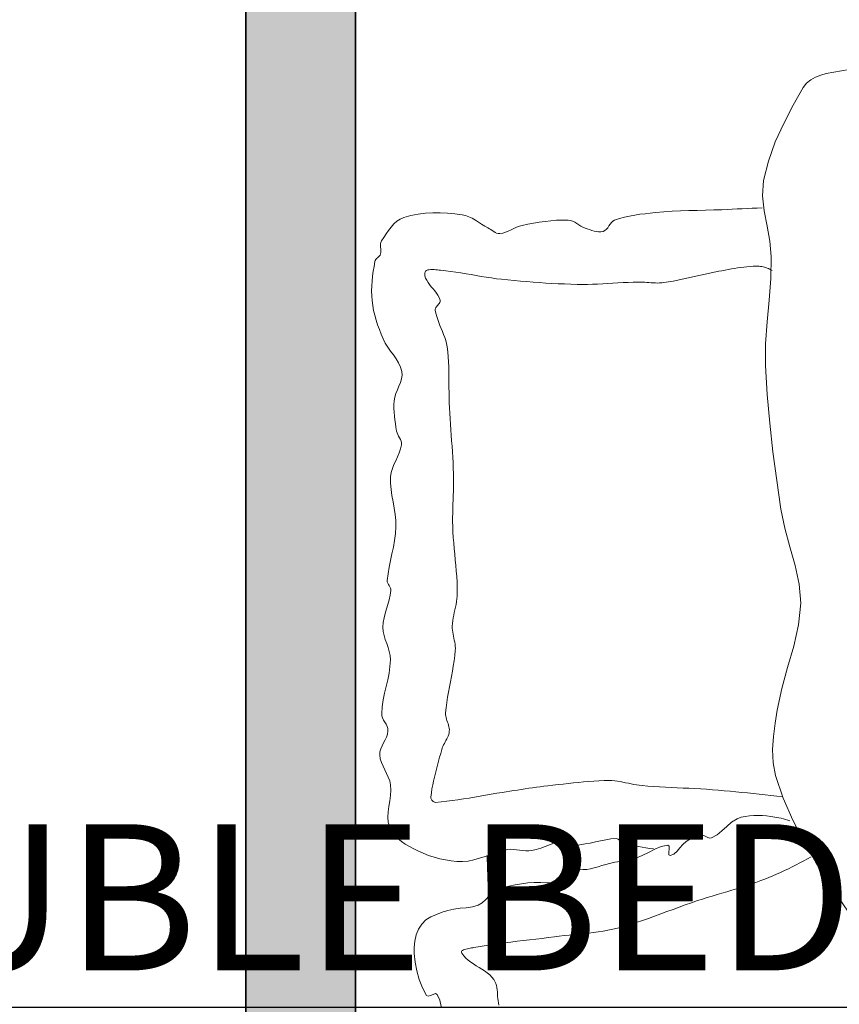
# Model space of a CAD drawing. Units: inches. Extents: x 2656 to 9931, y 1941 to 3068.
# Tile 16 of 46: x 2863 to 2896, y 2490 to 2530. Entities that reach past the tile are written whole.
import ezdxf

# ---------------------------------------------------------------- set-up
doc = ezdxf.new("R2010")
doc.units = ezdxf.units.IN
for name, color, linetype, lineweight in [('A-ANNO-DIMS', 2, 'Continuous', 18), ('A-FURN', 8, 'Continuous', 13), ('A-WALL', 7, 'Continuous', 35), ('A-WALL-PATT', 251, 'Continuous', 13)]:
    doc.layers.add(name, color=color, linetype=linetype, lineweight=lineweight)
doc.styles.get("Standard").update_dxf_attribs({"font": 'arial.ttf'})
doc.dimstyles.new('ISO-25', dxfattribs={"dimtxt": 6, "dimasz": 2.5, "dimexe": 1.25, "dimexo": 0.625, "dimtad": 1, "dimdec": 0, "dimlunit": 3, "dimtxsty": 'Standard', "dimcen": 2.5, "dimadec": 0, "dimazin": 0, "dimtfac": 1, "dimtdec": 0, "dimtmove": 0, "dimatfit": 3, "dimfxl": 1, "dimarcsym": 0})

# ---------------------------------------------------------------- blocks, each defined once
blk = doc.blocks.new('BED-DOUBLE')
for p, q in [((19.868, 60.758), (18.612, 60.54)), ((17.974, 60.285), (17.799, 60.142)), ((18.176, 60.399), (17.974, 60.285)), ((18.392, 60.483), (18.176, 60.399)), ((18.612, 60.54), (18.392, 60.483)), ((17.664, 59.967), (17.251, 59.242)), ((17.799, 60.142), (17.664, 59.967)), ((17.251, 59.242), (16.864, 58.499)), ((16.864, 58.499), (16.52, 57.736)), ((16.52, 57.736), (16.239, 56.953)), ((16.239, 56.953), (16.039, 56.149)), ((16.039, 56.149), (15.997, 55.53)), ((15.997, 55.53), (16.064, 54.908)), ((14.539, 54.965), (14.333, 54.956)), ((14.745, 54.974), (14.539, 54.965)), ((14.951, 54.984), (14.745, 54.974)), ((15.157, 54.993), (14.951, 54.984)), ((15.363, 55.002), (15.157, 54.993)), ((15.569, 55.012), (15.363, 55.002)), ((15.775, 55.021), (15.569, 55.012)), ((15.98, 55.031), (15.775, 55.021)), ((1.134, 54.573), (0.997, 54.482)), ((1.286, 54.638), (1.134, 54.573)), ((1.573, 54.718), (1.286, 54.638)), ((1.867, 54.773), (1.573, 54.718)), ((2.165, 54.807), (1.867, 54.773)), ((2.466, 54.823), (2.165, 54.807)), ((2.769, 54.822), (2.466, 54.823)), ((3.071, 54.807), (2.769, 54.822)), ((3.373, 54.782), (3.071, 54.807)), ((3.671, 54.748), (3.373, 54.782)), ((3.815, 54.718), (3.671, 54.748)), ((3.953, 54.668), (3.815, 54.718)), ((4.086, 54.602), (3.953, 54.668)), ((4.216, 54.525), (4.086, 54.602)), ((10.131, 54.589), (9.929, 54.522)), ((10.337, 54.645), (10.131, 54.589)), ((10.545, 54.692), (10.337, 54.645)), ((10.755, 54.732), (10.545, 54.692)), ((10.967, 54.765), (10.755, 54.732)), ((11.179, 54.792), (10.967, 54.765)), ((11.392, 54.817), (11.179, 54.792)), ((11.605, 54.838), (11.392, 54.817)), ((11.945, 54.867), (11.605, 54.838)), ((12.285, 54.889), (11.945, 54.867)), ((12.626, 54.904), (12.285, 54.889)), ((12.968, 54.916), (12.626, 54.904)), ((13.309, 54.925), (12.968, 54.916)), ((13.651, 54.933), (13.309, 54.925)), ((13.992, 54.943), (13.651, 54.933)), ((14.333, 54.956), (13.992, 54.943)), ((16.064, 54.908), (16.183, 54.283)), ((0.756, 54.244), (0.65, 54.106)), ((0.871, 54.371), (0.756, 54.244)), ((0.997, 54.482), (0.871, 54.371)), ((4.344, 54.443), (4.216, 54.525)), ((4.471, 54.359), (4.344, 54.443)), ((4.6, 54.279), (4.471, 54.359)), ((4.732, 54.207), (4.6, 54.279)), ((4.791, 54.174), (4.732, 54.207)), ((4.85, 54.136), (4.791, 54.174)), ((5.792, 54.184), (5.68, 54.13)), ((5.905, 54.235), (5.792, 54.184)), ((6.02, 54.279), (5.905, 54.235)), ((6.138, 54.31), (6.02, 54.279)), ((6.371, 54.355), (6.138, 54.31)), ((6.605, 54.399), (6.371, 54.355)), ((6.84, 54.439), (6.605, 54.399)), ((7.076, 54.474), (6.84, 54.439)), ((7.312, 54.503), (7.076, 54.474)), ((7.548, 54.522), (7.312, 54.503)), ((7.785, 54.531), (7.548, 54.522)), ((8.022, 54.528), (7.785, 54.531)), ((8.115, 54.514), (8.022, 54.528)), ((8.204, 54.483), (8.115, 54.514)), ((8.29, 54.44), (8.204, 54.483)), ((8.374, 54.39), (8.29, 54.44)), ((8.458, 54.336), (8.374, 54.39)), ((8.542, 54.284), (8.458, 54.336)), ((8.628, 54.237), (8.542, 54.284)), ((8.717, 54.201), (8.628, 54.237)), ((8.808, 54.17), (8.717, 54.201)), ((8.9, 54.138), (8.808, 54.17)), ((9.647, 54.214), (9.593, 54.149)), ((9.696, 54.287), (9.647, 54.214)), ((9.746, 54.36), (9.696, 54.287)), ((9.799, 54.428), (9.746, 54.36)), ((9.858, 54.484), (9.799, 54.428)), ((9.929, 54.522), (9.858, 54.484)), ((16.183, 54.283), (16.3, 53.657)), ((0.456, 53.815), (0.365, 53.671)), ((0.55, 53.961), (0.456, 53.815)), ((0.65, 54.106), (0.55, 53.961)), ((4.909, 54.096), (4.85, 54.136)), ((4.968, 54.058), (4.909, 54.096)), ((5.028, 54.024), (4.968, 54.058)), ((5.089, 53.997), (5.028, 54.024)), ((5.153, 53.981), (5.089, 53.997)), ((5.218, 53.978), (5.153, 53.981)), ((5.338, 53.997), (5.218, 53.978)), ((5.454, 54.031), (5.338, 53.997)), ((5.568, 54.077), (5.454, 54.031)), ((5.68, 54.13), (5.568, 54.077)), ((8.993, 54.107), (8.9, 54.138)), ((9.087, 54.08), (8.993, 54.107)), ((9.181, 54.059), (9.087, 54.08)), ((9.274, 54.048), (9.181, 54.059)), ((9.367, 54.049), (9.274, 54.048)), ((9.459, 54.064), (9.367, 54.049)), ((9.532, 54.097), (9.459, 54.064)), ((9.593, 54.149), (9.532, 54.097)), ((0.326, 53.548), (0.324, 53.481)), ((0.324, 53.481), (0.33, 53.412)), ((0.337, 53.612), (0.326, 53.548)), ((0.33, 53.412), (0.337, 53.342)), ((0.365, 53.671), (0.337, 53.612)), ((16.3, 53.657), (16.356, 53.03)), ((0.167, 52.946), (0.134, 52.909)), ((0.203, 52.982), (0.167, 52.946)), ((0.241, 53.017), (0.203, 52.982)), ((0.276, 53.054), (0.241, 53.017)), ((0.306, 53.094), (0.276, 53.054)), ((0.326, 53.138), (0.306, 53.094)), ((0.339, 53.203), (0.326, 53.138)), ((0.337, 53.342), (0.341, 53.272)), ((0.341, 53.272), (0.339, 53.203)), ((16.356, 53.03), (16.332, 52.135)), ((0.058, 52.625), (0.027, 52.426)), ((0.093, 52.823), (0.058, 52.625)), ((0.108, 52.868), (0.093, 52.823)), ((0.134, 52.909), (0.108, 52.868)), ((14.717, 52.521), (14.845, 52.543)), ((14.845, 52.543), (14.973, 52.563)), ((14.973, 52.563), (15.102, 52.582)), ((15.102, 52.582), (15.23, 52.599)), ((15.23, 52.599), (15.359, 52.614)), ((15.359, 52.614), (15.488, 52.625)), ((15.488, 52.625), (15.617, 52.633)), ((15.617, 52.633), (15.747, 52.637)), ((15.747, 52.637), (15.802, 52.637)), ((15.802, 52.637), (15.858, 52.634)), ((15.858, 52.634), (15.913, 52.628)), ((15.913, 52.628), (15.969, 52.619)), ((15.969, 52.619), (16.024, 52.608)), ((16.024, 52.608), (16.079, 52.595)), ((16.079, 52.595), (16.133, 52.579)), ((16.133, 52.579), (16.186, 52.561)), ((16.186, 52.561), (16.238, 52.54)), ((16.238, 52.54), (16.289, 52.517)), ((0, 52.226), (-0.022, 52.025)), ((0.027, 52.426), (0, 52.226)), ((2.14, 52.349), (2.15, 52.398)), ((2.149, 52.246), (2.14, 52.349)), ((2.176, 52.149), (2.149, 52.246)), ((2.15, 52.398), (2.175, 52.435)), ((2.175, 52.435), (2.213, 52.463)), ((2.219, 52.056), (2.176, 52.149)), ((2.213, 52.463), (2.262, 52.481)), ((2.262, 52.481), (2.32, 52.492)), ((2.32, 52.492), (2.384, 52.497)), ((2.384, 52.497), (2.453, 52.497)), ((2.453, 52.497), (2.525, 52.494)), ((2.525, 52.494), (2.597, 52.487)), ((2.597, 52.487), (2.666, 52.48)), ((2.666, 52.48), (2.731, 52.473)), ((2.731, 52.473), (2.79, 52.468)), ((2.79, 52.468), (3, 52.448)), ((3, 52.448), (3.209, 52.423)), ((3.209, 52.423), (3.417, 52.394)), ((3.417, 52.394), (3.625, 52.362)), ((3.625, 52.362), (3.833, 52.327)), ((3.833, 52.327), (4.041, 52.291)), ((4.041, 52.291), (4.248, 52.254)), ((4.248, 52.254), (4.456, 52.218)), ((4.456, 52.218), (4.664, 52.184)), ((4.664, 52.184), (4.872, 52.152)), ((4.872, 52.152), (5.081, 52.123)), ((12.705, 52.097), (12.892, 52.139)), ((12.892, 52.139), (13.08, 52.182)), ((13.08, 52.182), (13.267, 52.226)), ((13.267, 52.226), (13.454, 52.269)), ((13.454, 52.269), (13.641, 52.312)), ((13.641, 52.312), (13.829, 52.354)), ((13.829, 52.354), (14.017, 52.392)), ((14.017, 52.392), (14.206, 52.428)), ((14.206, 52.428), (14.333, 52.451)), ((14.333, 52.451), (14.461, 52.474)), ((14.461, 52.474), (14.589, 52.498)), ((14.589, 52.498), (14.717, 52.521)), ((16.332, 52.135), (16.264, 51.241)), ((16.289, 52.517), (16.338, 52.491)), ((16.338, 52.491), (16.386, 52.464)), ((-0.036, 51.824), (-0.042, 51.623)), ((-0.022, 52.025), (-0.036, 51.824)), ((2.274, 51.966), (2.219, 52.056)), ((2.338, 51.878), (2.274, 51.966)), ((2.408, 51.792), (2.338, 51.878)), ((2.481, 51.706), (2.408, 51.792)), ((5.081, 52.123), (5.29, 52.099)), ((5.29, 52.099), (5.548, 52.073)), ((5.548, 52.073), (5.806, 52.048)), ((5.806, 52.048), (6.065, 52.025)), ((6.065, 52.025), (6.323, 52.003)), ((6.323, 52.003), (6.582, 51.982)), ((6.582, 51.982), (6.841, 51.963)), ((6.841, 51.963), (7.1, 51.946)), ((7.1, 51.946), (7.359, 51.931)), ((7.359, 51.931), (7.618, 51.918)), ((7.618, 51.918), (7.877, 51.907)), ((7.877, 51.907), (8.136, 51.898)), ((8.136, 51.898), (8.396, 51.891)), ((8.396, 51.891), (8.604, 51.889)), ((8.604, 51.889), (8.813, 51.891)), ((8.813, 51.891), (9.022, 51.897)), ((9.022, 51.897), (9.231, 51.905)), ((9.231, 51.905), (9.44, 51.915)), ((9.44, 51.915), (9.648, 51.927)), ((9.648, 51.927), (9.857, 51.939)), ((9.857, 51.939), (10.066, 51.951)), ((10.066, 51.951), (10.275, 51.963)), ((10.275, 51.963), (10.483, 51.973)), ((10.483, 51.973), (10.692, 51.981)), ((10.692, 51.981), (10.901, 51.987)), ((10.901, 51.987), (10.989, 51.987)), ((10.989, 51.987), (11.076, 51.984)), ((11.076, 51.984), (11.164, 51.979)), ((11.164, 51.979), (11.251, 51.973)), ((11.251, 51.973), (11.339, 51.966)), ((11.339, 51.966), (11.427, 51.959)), ((11.427, 51.959), (11.514, 51.953)), ((11.514, 51.953), (11.601, 51.948)), ((11.601, 51.948), (11.689, 51.946)), ((11.689, 51.946), (11.776, 51.947)), ((11.776, 51.947), (11.863, 51.952)), ((11.863, 51.952), (11.95, 51.961)), ((11.95, 51.961), (12.14, 51.989)), ((12.14, 51.989), (12.329, 52.021)), ((12.329, 52.021), (12.517, 52.058)), ((12.517, 52.058), (12.705, 52.097)), ((-0.042, 51.623), (-0.038, 51.422)), ((-0.038, 51.422), (-0.022, 51.223)), ((2.552, 51.62), (2.481, 51.706)), ((2.62, 51.532), (2.552, 51.62)), ((2.681, 51.441), (2.62, 51.532)), ((2.731, 51.346), (2.681, 51.441)), ((2.768, 51.248), (2.731, 51.346)), ((-0.022, 51.223), (0.005, 51.02)), ((0.005, 51.02), (0.042, 50.82)), ((2.582, 50.904), (2.599, 50.939)), ((2.599, 50.939), (2.622, 50.973)), ((2.622, 50.973), (2.649, 51.007)), ((2.649, 51.007), (2.678, 51.041)), ((2.678, 51.041), (2.706, 51.074)), ((2.706, 51.074), (2.731, 51.108)), ((2.731, 51.108), (2.752, 51.141)), ((2.752, 51.141), (2.767, 51.176)), ((2.767, 51.176), (2.773, 51.211)), ((2.773, 51.211), (2.768, 51.248)), ((16.264, 51.241), (16.184, 50.347)), ((0.042, 50.82), (0.09, 50.62)), ((0.09, 50.62), (0.145, 50.423)), ((2.572, 50.868), (2.582, 50.904)), ((2.572, 50.83), (2.572, 50.868)), ((2.597, 50.702), (2.572, 50.83)), ((2.63, 50.575), (2.597, 50.702)), ((2.67, 50.45), (2.63, 50.575)), ((0.145, 50.423), (0.208, 50.227)), ((0.208, 50.227), (0.277, 50.034)), ((2.715, 50.326), (2.67, 50.45)), ((2.764, 50.203), (2.715, 50.326)), ((2.815, 50.081), (2.764, 50.203)), ((16.184, 50.347), (16.125, 49.453)), ((0.277, 50.034), (0.35, 49.842)), ((0.35, 49.842), (0.428, 49.653)), ((2.865, 49.958), (2.815, 50.081)), ((2.914, 49.835), (2.865, 49.958)), ((2.959, 49.711), (2.914, 49.835)), ((2.999, 49.586), (2.959, 49.711)), ((0.428, 49.653), (0.515, 49.48)), ((0.515, 49.48), (0.62, 49.315)), ((0.62, 49.315), (0.736, 49.155)), ((3.032, 49.459), (2.999, 49.586)), ((3.055, 49.331), (3.032, 49.459)), ((3.082, 49.123), (3.055, 49.331)), ((16.125, 49.453), (16.121, 48.558)), ((0.736, 49.155), (0.854, 48.996)), ((0.854, 48.996), (0.968, 48.836)), ((3.101, 48.916), (3.082, 49.123)), ((3.115, 48.707), (3.101, 48.916)), ((0.968, 48.836), (1.068, 48.671)), ((1.068, 48.671), (1.148, 48.498)), ((1.148, 48.498), (1.199, 48.315)), ((3.124, 48.499), (3.115, 48.707)), ((3.129, 48.29), (3.124, 48.499)), ((16.121, 48.558), (16.187, 47.374)), ((1.208, 48.162), (1.186, 48.011)), ((1.199, 48.315), (1.208, 48.162)), ((3.132, 48.081), (3.129, 48.29)), ((1.083, 47.712), (1.02, 47.562)), ((1.142, 47.861), (1.083, 47.712)), ((1.186, 48.011), (1.142, 47.861)), ((3.133, 47.871), (3.132, 48.081)), ((3.134, 47.662), (3.133, 47.871)), ((0.96, 47.411), (0.912, 47.259)), ((1.02, 47.562), (0.96, 47.411)), ((3.135, 47.452), (3.134, 47.662)), ((3.137, 47.243), (3.135, 47.452)), ((16.187, 47.374), (16.29, 46.193)), ((0.885, 47.105), (0.876, 46.95)), ((0.876, 46.95), (0.876, 46.796)), ((0.912, 47.259), (0.885, 47.105)), ((3.142, 47.034), (3.137, 47.243)), ((3.151, 46.825), (3.142, 47.034)), ((0.876, 46.796), (0.882, 46.641)), ((0.882, 46.641), (0.895, 46.486)), ((0.895, 46.486), (0.913, 46.331)), ((3.163, 46.599), (3.151, 46.825)), ((3.178, 46.373), (3.163, 46.599)), ((0.913, 46.331), (0.935, 46.177)), ((0.935, 46.177), (0.959, 46.023)), ((3.193, 46.147), (3.178, 46.373)), ((3.209, 45.922), (3.193, 46.147)), ((16.29, 46.193), (16.422, 45.014)), ((0.959, 46.023), (0.984, 45.87)), ((0.984, 45.87), (1.003, 45.798)), ((1.003, 45.798), (1.033, 45.727)), ((1.033, 45.727), (1.069, 45.658)), ((3.226, 45.696), (3.209, 45.922)), ((3.243, 45.47), (3.226, 45.696)), ((1.069, 45.658), (1.107, 45.59)), ((1.107, 45.59), (1.143, 45.521)), ((1.143, 45.521), (1.17, 45.452)), ((1.187, 45.308), (1.151, 45.139)), ((1.17, 45.452), (1.187, 45.381)), ((1.187, 45.381), (1.187, 45.308)), ((3.259, 45.245), (3.243, 45.47)), ((1.095, 44.974), (1.026, 44.812)), ((1.151, 45.139), (1.095, 44.974)), ((3.275, 45.019), (3.259, 45.245)), ((3.289, 44.793), (3.275, 45.019)), ((16.422, 45.014), (16.577, 43.838)), ((0.877, 44.491), (0.812, 44.328)), ((0.951, 44.651), (0.877, 44.491)), ((1.026, 44.812), (0.951, 44.651)), ((3.302, 44.567), (3.289, 44.793)), ((3.312, 44.341), (3.302, 44.567)), ((0.763, 44.162), (0.738, 43.992)), ((0.812, 44.328), (0.763, 44.162)), ((3.32, 44.115), (3.312, 44.341)), ((3.323, 43.936), (3.32, 44.115)), ((0.738, 43.992), (0.735, 43.734)), ((0.735, 43.734), (0.756, 43.477)), ((3.32, 43.578), (3.323, 43.757)), ((3.323, 43.757), (3.323, 43.936)), ((16.577, 43.838), (16.745, 42.664)), ((0.756, 43.477), (0.793, 43.221)), ((3.309, 43.22), (3.315, 43.399)), ((3.315, 43.399), (3.32, 43.578)), ((0.793, 43.221), (0.839, 42.964)), ((0.839, 42.964), (0.887, 42.708)), ((3.289, 42.683), (3.295, 42.862)), ((3.295, 42.862), (3.302, 43.041)), ((3.302, 43.041), (3.309, 43.22)), ((0.887, 42.708), (0.928, 42.451)), ((0.928, 42.451), (0.954, 42.194)), ((3.282, 42.325), (3.285, 42.504)), ((3.285, 42.504), (3.289, 42.683)), ((16.745, 42.664), (16.906, 41.889)), ((0.954, 42.194), (0.959, 41.936)), ((3.283, 42.146), (3.282, 42.325)), ((3.286, 41.967), (3.283, 42.146)), ((0.94, 41.658), (0.902, 41.381)), ((0.959, 41.936), (0.94, 41.658)), ((3.296, 41.737), (3.286, 41.967)), ((3.311, 41.506), (3.296, 41.737)), ((16.906, 41.889), (17.122, 41.121)), ((0.902, 41.381), (0.851, 41.106)), ((3.328, 41.276), (3.311, 41.506)), ((3.349, 41.046), (3.328, 41.276)), ((0.794, 40.832), (0.734, 40.557)), ((0.851, 41.106), (0.794, 40.832)), ((3.371, 40.816), (3.349, 41.046)), ((17.122, 41.121), (17.339, 40.355)), ((0.734, 40.557), (0.679, 40.282)), ((3.393, 40.587), (3.371, 40.816)), ((3.414, 40.357), (3.393, 40.587)), ((0.679, 40.282), (0.633, 40.006)), ((3.434, 40.127), (3.414, 40.357)), ((3.45, 39.897), (3.434, 40.127)), ((17.339, 40.355), (17.503, 39.584)), ((0.633, 40.006), (0.601, 39.729)), ((0.601, 39.729), (0.604, 39.676)), ((0.604, 39.676), (0.621, 39.624)), ((0.621, 39.624), (0.646, 39.574)), ((3.464, 39.667), (3.45, 39.897)), ((3.472, 39.436), (3.464, 39.667)), ((0.646, 39.574), (0.675, 39.524)), ((0.675, 39.524), (0.704, 39.474)), ((0.704, 39.474), (0.729, 39.424)), ((0.748, 39.32), (0.721, 39.13)), ((0.729, 39.424), (0.745, 39.373)), ((0.745, 39.373), (0.748, 39.32)), ((3.469, 39.093), (3.474, 39.206)), ((3.474, 39.206), (3.472, 39.436)), ((17.503, 39.584), (17.561, 38.802)), ((0.678, 38.942), (0.626, 38.755)), ((0.721, 39.13), (0.678, 38.942)), ((3.422, 38.756), (3.443, 38.868)), ((3.443, 38.868), (3.459, 38.98)), ((3.459, 38.98), (3.469, 39.093)), ((17.561, 38.802), (17.472, 37.913)), ((0.57, 38.57), (0.516, 38.384)), ((0.626, 38.755), (0.57, 38.57)), ((3.326, 38.31), (3.35, 38.422)), ((3.35, 38.422), (3.375, 38.533)), ((3.375, 38.533), (3.399, 38.645)), ((3.399, 38.645), (3.422, 38.756)), ((0.437, 38.008), (0.424, 37.818)), ((0.469, 38.197), (0.437, 38.008)), ((0.516, 38.384), (0.469, 38.197)), ((3.273, 37.974), (3.287, 38.087)), ((3.287, 38.087), (3.305, 38.199)), ((3.305, 38.199), (3.326, 38.31)), ((0.424, 37.818), (0.437, 37.648)), ((0.437, 37.648), (0.472, 37.481)), ((3.266, 37.861), (3.273, 37.974)), ((3.267, 37.778), (3.266, 37.861)), ((3.273, 37.695), (3.267, 37.778)), ((3.285, 37.612), (3.273, 37.695)), ((3.3, 37.529), (3.285, 37.612)), ((17.472, 37.913), (17.275, 37.038)), ((0.472, 37.481), (0.522, 37.316)), ((0.522, 37.316), (0.579, 37.151)), ((3.317, 37.447), (3.3, 37.529)), ((3.335, 37.364), (3.317, 37.447)), ((3.353, 37.282), (3.335, 37.364)), ((3.369, 37.199), (3.353, 37.282)), ((3.383, 37.116), (3.369, 37.199)), ((0.579, 37.151), (0.636, 36.987)), ((0.636, 36.987), (0.686, 36.822)), ((0.686, 36.822), (0.72, 36.655)), ((3.373, 36.652), (3.393, 36.868)), ((3.392, 37.034), (3.383, 37.116)), ((3.396, 36.951), (3.392, 37.034)), ((3.393, 36.868), (3.396, 36.951)), ((17.275, 37.038), (17.026, 36.168)), ((0.731, 36.485), (0.714, 36.207)), ((0.72, 36.655), (0.731, 36.485)), ((3.312, 36.223), (3.345, 36.437)), ((3.345, 36.437), (3.373, 36.652)), ((0.714, 36.207), (0.674, 35.931)), ((3.234, 35.796), (3.274, 36.01)), ((3.274, 36.01), (3.312, 36.223)), ((17.026, 36.168), (16.783, 35.296)), ((0.62, 35.656), (0.558, 35.381)), ((0.674, 35.931), (0.62, 35.656)), ((3.15, 35.37), (3.192, 35.583)), ((3.192, 35.583), (3.234, 35.796)), ((0.558, 35.381), (0.495, 35.107)), ((3.11, 35.157), (3.15, 35.37)), ((16.783, 35.296), (16.603, 34.415)), ((0.438, 34.832), (0.395, 34.556)), ((0.495, 35.107), (0.438, 34.832)), ((3.039, 34.729), (3.072, 34.943)), ((3.072, 34.943), (3.11, 35.157)), ((0.395, 34.556), (0.373, 34.278)), ((2.992, 34.298), (3.012, 34.514)), ((3.012, 34.514), (3.039, 34.729)), ((16.603, 34.415), (16.521, 33.879)), ((0.373, 34.278), (0.382, 34.185)), ((0.382, 34.185), (0.411, 34.095)), ((0.411, 34.095), (0.454, 34.007)), ((0.454, 34.007), (0.503, 33.92)), ((2.992, 34.235), (2.992, 34.298)), ((2.999, 34.172), (2.992, 34.235)), ((3.012, 34.109), (2.999, 34.172)), ((3.03, 34.047), (3.012, 34.109)), ((3.05, 33.984), (3.03, 34.047)), ((3.073, 33.922), (3.05, 33.984)), ((0.503, 33.92), (0.552, 33.833)), ((0.552, 33.833), (0.594, 33.745)), ((0.594, 33.745), (0.623, 33.655)), ((0.631, 33.562), (0.611, 33.435)), ((0.623, 33.655), (0.631, 33.562)), ((3.095, 33.86), (3.073, 33.922)), ((3.115, 33.798), (3.095, 33.86)), ((3.132, 33.736), (3.115, 33.798)), ((3.144, 33.673), (3.132, 33.736)), ((3.137, 33.48), (3.148, 33.546)), ((3.15, 33.61), (3.144, 33.673)), ((3.148, 33.546), (3.15, 33.61)), ((16.521, 33.879), (16.449, 33.336)), ((0.513, 33.189), (0.45, 33.069)), ((0.569, 33.31), (0.513, 33.189)), ((0.611, 33.435), (0.569, 33.31)), ((2.978, 33.11), (3.011, 33.17)), ((3.011, 33.17), (3.042, 33.231)), ((3.042, 33.231), (3.072, 33.292)), ((3.072, 33.292), (3.098, 33.353)), ((3.098, 33.353), (3.121, 33.416)), ((3.121, 33.416), (3.137, 33.48)), ((16.449, 33.336), (16.409, 32.793)), ((0.337, 32.827), (0.303, 32.703)), ((0.389, 32.949), (0.337, 32.827)), ((0.45, 33.069), (0.389, 32.949)), ((2.794, 32.639), (2.84, 32.8)), ((2.84, 32.8), (2.86, 32.864)), ((2.86, 32.864), (2.886, 32.927)), ((2.886, 32.927), (2.915, 32.989)), ((2.915, 32.989), (2.946, 33.049)), ((2.946, 33.049), (2.978, 33.11)), ((16.409, 32.793), (16.428, 32.257)), ((0.303, 32.703), (0.294, 32.575)), ((0.294, 32.575), (0.317, 32.415)), ((0.317, 32.415), (0.364, 32.261)), ((2.704, 32.317), (2.749, 32.479)), ((2.749, 32.479), (2.794, 32.639)), ((0.364, 32.261), (0.428, 32.11)), ((0.428, 32.11), (0.501, 31.961)), ((0.501, 31.961), (0.576, 31.812)), ((2.576, 31.832), (2.617, 31.994)), ((2.617, 31.994), (2.66, 32.156)), ((2.66, 32.156), (2.704, 32.317)), ((16.428, 32.257), (16.53, 31.734)), ((0.576, 31.812), (0.645, 31.661)), ((0.645, 31.661), (0.701, 31.508)), ((2.5, 31.506), (2.537, 31.669)), ((2.537, 31.669), (2.576, 31.832)), ((9.707, 31.525), (9.497, 31.522)), ((9.821, 31.521), (9.707, 31.525)), ((16.53, 31.734), (16.849, 30.803)), ((0.701, 31.508), (0.736, 31.349)), ((0.748, 31.131), (0.733, 30.909)), ((0.736, 31.349), (0.748, 31.131)), ((2.411, 31.014), (2.437, 31.178)), ((2.437, 31.178), (2.467, 31.343)), ((2.467, 31.343), (2.5, 31.506)), ((5.943, 31.135), (5.788, 31.111)), ((6.098, 31.159), (5.943, 31.135)), ((6.254, 31.183), (6.098, 31.159)), ((6.409, 31.206), (6.254, 31.183)), ((6.564, 31.229), (6.409, 31.206)), ((6.72, 31.25), (6.564, 31.229)), ((6.876, 31.271), (6.72, 31.25)), ((7.031, 31.291), (6.876, 31.271)), ((7.188, 31.309), (7.031, 31.291)), ((7.397, 31.332), (7.188, 31.309)), ((7.607, 31.357), (7.397, 31.332)), ((7.816, 31.381), (7.607, 31.357)), ((8.026, 31.405), (7.816, 31.381)), ((8.236, 31.429), (8.026, 31.405)), ((8.446, 31.451), (8.236, 31.429)), ((8.656, 31.471), (8.446, 31.451)), ((8.866, 31.488), (8.656, 31.471)), ((9.076, 31.503), (8.866, 31.488)), ((9.286, 31.514), (9.076, 31.503)), ((9.497, 31.522), (9.286, 31.514)), ((9.933, 31.512), (9.821, 31.521)), ((10.045, 31.498), (9.933, 31.512)), ((10.157, 31.48), (10.045, 31.498)), ((10.269, 31.459), (10.157, 31.48)), ((10.381, 31.436), (10.269, 31.459)), ((10.492, 31.412), (10.381, 31.436)), ((10.604, 31.389), (10.492, 31.412)), ((10.715, 31.366), (10.604, 31.389)), ((10.827, 31.346), (10.715, 31.366)), ((10.94, 31.329), (10.827, 31.346)), ((11.052, 31.317), (10.94, 31.329)), ((11.293, 31.297), (11.052, 31.317)), ((11.533, 31.28), (11.293, 31.297)), ((11.774, 31.265), (11.533, 31.28)), ((12.015, 31.252), (11.774, 31.265)), ((12.256, 31.24), (12.015, 31.252)), ((12.497, 31.228), (12.256, 31.24)), ((12.738, 31.217), (12.497, 31.228)), ((12.979, 31.206), (12.738, 31.217)), ((13.22, 31.194), (12.979, 31.206)), ((13.461, 31.18), (13.22, 31.194)), ((13.702, 31.165), (13.461, 31.18)), ((13.942, 31.147), (13.702, 31.165)), ((14.182, 31.127), (13.942, 31.147)), ((14.422, 31.107), (14.182, 31.127)), ((0.733, 30.909), (0.701, 30.686)), ((2.389, 30.848), (2.411, 31.014)), ((2.389, 30.823), (2.389, 30.848)), ((2.393, 30.798), (2.389, 30.823)), ((2.401, 30.772), (2.393, 30.798)), ((2.413, 30.747), (2.401, 30.772)), ((2.428, 30.723), (2.413, 30.747)), ((2.445, 30.7), (2.428, 30.723)), ((3.5, 30.733), (3.271, 30.7)), ((3.728, 30.769), (3.5, 30.733)), ((3.955, 30.807), (3.728, 30.769)), ((4.183, 30.847), (3.955, 30.807)), ((4.411, 30.887), (4.183, 30.847)), ((4.638, 30.927), (4.411, 30.887)), ((4.866, 30.967), (4.638, 30.927)), ((5.094, 31.005), (4.866, 30.967)), ((5.322, 31.04), (5.094, 31.005)), ((5.477, 31.063), (5.322, 31.04)), ((5.632, 31.087), (5.477, 31.063)), ((5.788, 31.111), (5.632, 31.087)), ((14.662, 31.085), (14.422, 31.107)), ((14.902, 31.063), (14.662, 31.085)), ((15.142, 31.04), (14.902, 31.063)), ((15.382, 31.016), (15.142, 31.04)), ((15.621, 30.992), (15.382, 31.016)), ((15.861, 30.966), (15.621, 30.992)), ((16.1, 30.94), (15.861, 30.966)), ((16.34, 30.913), (16.1, 30.94)), ((16.579, 30.885), (16.34, 30.913)), ((16.818, 30.856), (16.579, 30.885)), ((16.849, 30.803), (17.238, 29.898)), ((0.665, 30.462), (0.636, 30.241)), ((0.701, 30.686), (0.665, 30.462)), ((2.465, 30.68), (2.445, 30.7)), ((2.487, 30.662), (2.465, 30.68)), ((2.51, 30.647), (2.487, 30.662)), ((2.534, 30.637), (2.51, 30.647)), ((2.559, 30.631), (2.534, 30.637)), ((2.583, 30.63), (2.559, 30.631)), ((2.813, 30.648), (2.583, 30.63)), ((3.042, 30.672), (2.813, 30.648)), ((3.271, 30.7), (3.042, 30.672)), ((0.636, 30.241), (0.624, 30.023)), ((0.624, 30.023), (0.642, 29.81)), ((14.729, 29.815), (14.951, 29.952)), ((14.951, 29.952), (15.115, 30.015)), ((15.115, 30.015), (15.288, 30.055)), ((15.288, 30.055), (15.465, 30.077)), ((15.465, 30.077), (15.645, 30.088)), ((15.645, 30.088), (15.823, 30.093)), ((15.823, 30.093), (15.993, 30.09)), ((15.993, 30.09), (16.162, 30.075)), ((16.162, 30.075), (16.331, 30.052)), ((16.331, 30.052), (16.5, 30.023)), ((16.5, 30.023), (16.667, 29.993)), ((16.667, 29.993), (16.759, 29.975)), ((16.759, 29.975), (16.85, 29.954)), ((16.85, 29.954), (16.94, 29.928)), ((16.94, 29.928), (17.029, 29.899)), ((0.642, 29.81), (0.701, 29.605)), ((0.701, 29.605), (0.788, 29.438)), ((14.332, 29.466), (14.528, 29.645)), ((14.528, 29.645), (14.729, 29.815)), ((17.029, 29.899), (17.117, 29.867)), ((17.238, 29.898), (17.685, 29.016)), ((0.788, 29.438), (0.899, 29.287)), ((0.899, 29.287), (1.032, 29.151)), ((1.032, 29.151), (1.182, 29.027)), ((7.794, 29.077), (7.98, 29.112)), ((7.98, 29.112), (8.025, 29.107)), ((8.025, 29.107), (8.065, 29.082)), ((9.563, 29.094), (9.775, 29.126)), ((9.775, 29.126), (9.989, 29.144)), ((9.989, 29.144), (10.03, 29.139)), ((10.03, 29.139), (10.068, 29.122)), ((10.068, 29.122), (10.104, 29.096)), ((12.971, 29.097), (13.085, 29.165)), ((13.085, 29.165), (13.204, 29.223)), ((13.204, 29.223), (13.327, 29.269)), ((13.327, 29.269), (13.455, 29.297)), ((13.455, 29.297), (13.547, 29.286)), ((13.547, 29.286), (13.639, 29.244)), ((13.639, 29.244), (13.729, 29.194)), ((13.729, 29.194), (13.818, 29.162)), ((13.818, 29.162), (13.905, 29.17)), ((13.905, 29.17), (14.129, 29.301)), ((14.129, 29.301), (14.332, 29.466)), ((1.182, 29.027), (1.343, 28.914)), ((1.343, 28.914), (1.513, 28.813)), ((1.513, 28.813), (1.686, 28.721)), ((1.686, 28.721), (1.859, 28.637)), ((5.533, 28.692), (5.657, 28.702)), ((5.657, 28.702), (5.782, 28.699)), ((5.782, 28.699), (5.907, 28.685)), ((6.716, 28.689), (6.897, 28.747)), ((6.897, 28.747), (7.076, 28.815)), ((7.076, 28.815), (7.254, 28.887)), ((7.254, 28.887), (7.432, 28.958)), ((7.432, 28.958), (7.611, 29.024)), ((7.611, 29.024), (7.794, 29.077)), ((8.065, 29.082), (8.102, 29.045)), ((8.102, 29.045), (8.137, 29.001)), ((8.137, 29.001), (8.172, 28.956)), ((8.172, 28.956), (8.208, 28.917)), ((8.208, 28.917), (8.249, 28.889)), ((8.249, 28.889), (8.295, 28.879)), ((8.295, 28.879), (8.508, 28.892)), ((8.508, 28.892), (8.72, 28.921)), ((8.72, 28.921), (8.931, 28.961)), ((8.931, 28.961), (9.142, 29.006)), ((9.142, 29.006), (9.352, 29.052)), ((9.352, 29.052), (9.563, 29.094)), ((10.104, 29.096), (10.138, 29.066)), ((10.138, 29.066), (10.173, 29.034)), ((10.173, 29.034), (10.208, 29.004)), ((10.208, 29.004), (10.245, 28.979)), ((10.245, 28.979), (10.285, 28.962)), ((10.285, 28.962), (10.438, 28.921)), ((10.438, 28.921), (10.592, 28.883)), ((10.592, 28.883), (10.747, 28.848)), ((10.747, 28.848), (10.902, 28.816)), ((10.902, 28.816), (11.058, 28.787)), ((11.058, 28.787), (11.214, 28.761)), ((11.214, 28.761), (11.371, 28.738)), ((11.318, 28.576), (11.574, 28.708)), ((11.371, 28.738), (11.528, 28.717)), ((11.574, 28.708), (11.835, 28.814)), ((11.835, 28.814), (12.108, 28.869)), ((12.108, 28.869), (12.16, 28.826)), ((12.164, 28.715), (12.151, 28.582)), ((12.16, 28.826), (12.164, 28.715)), ((12.49, 28.625), (12.608, 28.765)), ((12.608, 28.765), (12.727, 28.906)), ((12.727, 28.906), (12.86, 29.025)), ((12.86, 29.025), (12.971, 29.097)), ((17.685, 29.016), (18.177, 28.157)), ((1.859, 28.637), (2.075, 28.541)), ((2.075, 28.541), (2.296, 28.454)), ((2.296, 28.454), (2.522, 28.379)), ((2.522, 28.379), (2.752, 28.315)), ((2.752, 28.315), (2.985, 28.264)), ((4.158, 28.267), (4.387, 28.334)), ((4.387, 28.334), (4.615, 28.412)), ((4.615, 28.412), (4.842, 28.495)), ((4.7, 28.368), (4.698, 28.448)), ((4.703, 28.288), (4.7, 28.368)), ((4.842, 28.495), (5.07, 28.574)), ((5.07, 28.574), (5.3, 28.643)), ((5.3, 28.643), (5.533, 28.692)), ((5.907, 28.685), (6.032, 28.668)), ((6.032, 28.668), (6.158, 28.65)), ((6.158, 28.65), (6.283, 28.638)), ((6.283, 28.638), (6.407, 28.635)), ((6.407, 28.635), (6.531, 28.647)), ((6.531, 28.647), (6.716, 28.689)), ((10.586, 28.283), (10.798, 28.339)), ((10.798, 28.339), (11.062, 28.445)), ((11.062, 28.445), (11.318, 28.576)), ((12.151, 28.582), (12.154, 28.476)), ((12.154, 28.476), (12.205, 28.442)), ((12.205, 28.442), (12.36, 28.509)), ((12.36, 28.509), (12.49, 28.625)), ((17.686, 28.224), (17.841, 28.308)), ((17.841, 28.308), (17.995, 28.394)), ((2.985, 28.264), (3.219, 28.227)), ((3.219, 28.227), (3.455, 28.205)), ((3.455, 28.205), (3.69, 28.2)), ((3.69, 28.2), (3.926, 28.22)), ((3.926, 28.22), (4.158, 28.267)), ((4.706, 28.209), (4.703, 28.288)), ((4.709, 28.129), (4.706, 28.209)), ((4.712, 28.049), (4.709, 28.129)), ((4.715, 27.969), (4.712, 28.049)), ((4.717, 27.889), (4.715, 27.969)), ((4.72, 27.81), (4.717, 27.889)), ((8.782, 27.876), (8.937, 27.898)), ((8.937, 27.898), (9.095, 27.938)), ((9.095, 27.938), (9.252, 27.984)), ((9.252, 27.984), (9.408, 28.034)), ((9.408, 28.034), (9.564, 28.082)), ((9.564, 28.082), (9.721, 28.124)), ((9.721, 28.124), (9.937, 28.168)), ((9.937, 28.168), (10.154, 28.204)), ((10.154, 28.204), (10.371, 28.24)), ((10.371, 28.24), (10.586, 28.283)), ((16.897, 27.83), (17.056, 27.905)), ((17.056, 27.905), (17.215, 27.982)), ((17.215, 27.982), (17.373, 28.061)), ((17.373, 28.061), (17.53, 28.142)), ((17.53, 28.142), (17.686, 28.224)), ((18.177, 28.157), (18.699, 27.32)), ((4.723, 27.73), (4.72, 27.81)), ((4.726, 27.65), (4.723, 27.73)), ((4.728, 27.57), (4.726, 27.65)), ((4.731, 27.49), (4.728, 27.57)), ((4.734, 27.41), (4.731, 27.49)), ((7.789, 27.442), (7.882, 27.53)), ((7.882, 27.53), (7.969, 27.632)), ((7.969, 27.632), (8.06, 27.726)), ((8.06, 27.726), (8.166, 27.794)), ((8.166, 27.794), (8.314, 27.837)), ((8.314, 27.837), (8.468, 27.857)), ((8.468, 27.857), (8.625, 27.867)), ((8.625, 27.867), (8.782, 27.876)), ((16.087, 27.48), (16.25, 27.546)), ((16.25, 27.546), (16.413, 27.614)), ((16.413, 27.614), (16.575, 27.684)), ((16.575, 27.684), (16.736, 27.756)), ((16.736, 27.756), (16.897, 27.83)), ((4.737, 27.331), (4.734, 27.41)), ((4.74, 27.251), (4.737, 27.331)), ((4.743, 27.171), (4.74, 27.251)), ((4.745, 27.091), (4.743, 27.171)), ((4.748, 27.011), (4.745, 27.091)), ((5.093, 27.032), (5.338, 27.125)), ((5.338, 27.125), (5.592, 27.193)), ((5.592, 27.193), (5.851, 27.245)), ((5.851, 27.245), (6.113, 27.285)), ((6.113, 27.285), (6.374, 27.321)), ((6.374, 27.321), (6.635, 27.34)), ((6.635, 27.34), (6.898, 27.338)), ((6.898, 27.338), (7.162, 27.333)), ((7.162, 27.333), (7.422, 27.343)), ((7.422, 27.343), (7.678, 27.387)), ((7.678, 27.387), (7.789, 27.442)), ((14.733, 27.021), (14.933, 27.081)), ((14.933, 27.081), (15.133, 27.143)), ((15.133, 27.143), (15.332, 27.207)), ((15.332, 27.207), (15.53, 27.273)), ((15.53, 27.273), (15.727, 27.343)), ((15.727, 27.343), (15.923, 27.416)), ((15.923, 27.416), (16.087, 27.48)), ((18.699, 27.32), (19.702, 25.863)), ((4.646, 26.646), (4.784, 26.793)), ((4.751, 26.932), (4.748, 27.011)), ((4.754, 26.852), (4.751, 26.932)), ((4.784, 26.793), (4.929, 26.929)), ((4.929, 26.929), (5.093, 27.032)), ((13.531, 26.661), (13.73, 26.724)), ((13.73, 26.724), (13.93, 26.784)), ((13.93, 26.784), (14.131, 26.844)), ((14.131, 26.844), (14.332, 26.903)), ((14.332, 26.903), (14.532, 26.961)), ((14.532, 26.961), (14.733, 27.021)), ((3.333, 26.252), (3.587, 26.281)), ((3.587, 26.281), (3.842, 26.303)), ((3.842, 26.303), (4.094, 26.34)), ((4.094, 26.34), (4.335, 26.412)), ((4.335, 26.412), (4.501, 26.512)), ((4.501, 26.512), (4.646, 26.646)), ((12.324, 26.237), (12.575, 26.33)), ((12.575, 26.33), (12.826, 26.422)), ((12.826, 26.422), (13.078, 26.511)), ((13.078, 26.511), (13.332, 26.597)), ((13.332, 26.597), (13.531, 26.661)), ((2.187, 25.802), (2.391, 25.931)), ((2.391, 25.931), (2.617, 26.032)), ((2.617, 26.032), (2.853, 26.116)), ((2.853, 26.116), (3.086, 26.193)), ((3.086, 26.193), (3.333, 26.252)), ((11.067, 25.778), (11.319, 25.866)), ((11.319, 25.866), (11.571, 25.957)), ((11.571, 25.957), (11.822, 26.049)), ((11.822, 26.049), (12.073, 26.143)), ((12.073, 26.143), (12.324, 26.237)), ((1.884, 25.422), (2.018, 25.634)), ((2.018, 25.634), (2.187, 25.802)), ((9.849, 25.423), (10.044, 25.469)), ((10.044, 25.469), (10.302, 25.538)), ((10.302, 25.538), (10.558, 25.613)), ((10.558, 25.613), (10.813, 25.693)), ((10.813, 25.693), (11.067, 25.778)), ((1.729, 24.935), (1.788, 25.186)), ((1.788, 25.186), (1.884, 25.422)), ((6.95, 25.048), (7.204, 25.081)), ((7.204, 25.081), (7.459, 25.114)), ((7.459, 25.114), (7.658, 25.139)), ((7.658, 25.139), (7.858, 25.162)), ((7.858, 25.162), (8.058, 25.184)), ((8.058, 25.184), (8.258, 25.204)), ((8.258, 25.204), (8.458, 25.224)), ((8.458, 25.224), (8.658, 25.245)), ((8.658, 25.245), (8.858, 25.267)), ((8.858, 25.267), (9.058, 25.291)), ((9.058, 25.291), (9.257, 25.318)), ((9.257, 25.318), (9.455, 25.348)), ((9.455, 25.348), (9.652, 25.383)), ((9.652, 25.383), (9.849, 25.423)), ((1.701, 24.678), (1.729, 24.935)), ((1.704, 24.424), (1.701, 24.678)), ((4.002, 24.647), (4.058, 24.657)), ((4.058, 24.657), (4.109, 24.665)), ((4.109, 24.665), (4.154, 24.673)), ((4.154, 24.673), (4.407, 24.716)), ((4.407, 24.716), (4.66, 24.756)), ((4.66, 24.756), (4.914, 24.794)), ((4.914, 24.794), (5.168, 24.829)), ((5.168, 24.829), (5.422, 24.863)), ((5.422, 24.863), (5.676, 24.895)), ((5.676, 24.895), (5.931, 24.926)), ((5.931, 24.926), (6.186, 24.957)), ((6.186, 24.957), (6.44, 24.987)), ((6.44, 24.987), (6.695, 25.017)), ((6.695, 25.017), (6.95, 25.048)), ((1.743, 24.066), (1.704, 24.424)), ((3.648, 24.471), (3.65, 24.502)), ((3.662, 24.438), (3.648, 24.471)), ((3.65, 24.502), (3.667, 24.529)), ((3.737, 24.332), (3.662, 24.438)), ((3.667, 24.529), (3.695, 24.553)), ((3.695, 24.553), (3.733, 24.574)), ((3.733, 24.574), (3.779, 24.593)), ((3.825, 24.237), (3.737, 24.332)), ((3.779, 24.593), (3.831, 24.609)), ((3.831, 24.609), (3.887, 24.623)), ((3.887, 24.623), (3.945, 24.636)), ((3.945, 24.636), (4.002, 24.647)), ((1.814, 23.71), (1.743, 24.066)), ((3.922, 24.151), (3.825, 24.237)), ((4.027, 24.071), (3.922, 24.151)), ((4.138, 23.996), (4.027, 24.071)), ((4.252, 23.924), (4.138, 23.996)), ((4.367, 23.854), (4.252, 23.924)), ((4.482, 23.783), (4.367, 23.854)), ((1.915, 23.361), (1.814, 23.71)), ((4.594, 23.709), (4.482, 23.783)), ((4.702, 23.631), (4.594, 23.709)), ((4.803, 23.547), (4.702, 23.631)), ((4.895, 23.455), (4.803, 23.547)), ((4.976, 23.353), (4.895, 23.455)), ((2.047, 23.023), (1.915, 23.361)), ((5.021, 23.278), (4.976, 23.353)), ((5.055, 23.198), (5.021, 23.278)), ((5.08, 23.115), (5.055, 23.198)), ((5.098, 23.029), (5.08, 23.115)), ((2.209, 22.702), (2.047, 23.023)), ((2.277, 22.669), (2.209, 22.702)), ((2.376, 22.698), (2.277, 22.669)), ((2.486, 22.749), (2.376, 22.698)), ((2.586, 22.779), (2.486, 22.749)), ((2.655, 22.747), (2.586, 22.779)), ((2.758, 22.509), (2.655, 22.747)), ((5.11, 22.94), (5.098, 23.029)), ((5.118, 22.85), (5.11, 22.94)), ((5.124, 22.758), (5.118, 22.85)), ((5.129, 22.666), (5.124, 22.758)), ((5.136, 22.575), (5.129, 22.666)), ((2.814, 22.253), (2.758, 22.509)), ((5.146, 22.484), (5.136, 22.575)), ((5.16, 22.395), (5.146, 22.484)), ((5.181, 22.309), (5.16, 22.395))]:
    blk.add_line(p, q)
blk = doc.blocks.new('*D31')
at = {"layer": 'A-ANNO-DIMS', "color": 0, "lineweight": -2, "transparency": 16777216}
for p, q in [((2753.358, 2502.145), (2753.358, 2488.227)), ((2841.982, 2502.145), (2841.982, 2488.227)), ((2755.858, 2489.477), (2839.482, 2489.477)), ((2841.982, 2489.477), (2952.348, 2489.477))]:
    blk.add_line(p, q, dxfattribs=at)
at = {"layer": 'A-ANNO-DIMS', "color": 0, "transparency": 16777216}
for points in [[(2755.858, 2489.893), (2755.858, 2489.06), (2753.358, 2489.477)], [(2839.482, 2489.893), (2839.482, 2489.06), (2841.982, 2489.477)]]:
    blk.add_solid(points, dxfattribs=at)
at = {"layer": 'Defpoints', "color": 0, "transparency": 16777216}
for p in [(2753.358, 2502.77), (2841.982, 2502.77), (2841.982, 2489.477)]:
    blk.add_point(p, dxfattribs=at)
at = {"layer": 'A-ANNO-DIMS', "color": 0, "transparency": 16777216, "insert": (2898.415, 2493.206), "char_height": 6, "attachment_point": 5}
blk.add_mtext('DOUBLE BED 7\'-4 1/2" TYP.', dxfattribs=at)
blk = doc.blocks.new('*D32')
at = {"layer": 'A-ANNO-DIMS', "color": 0, "lineweight": -2, "transparency": 16777216}
for p, q in [((2842.607, 2565.211), (2856.525, 2565.211)), ((2855.275, 2505.27), (2855.275, 2562.711)), ((2842.607, 2502.77), (2856.525, 2502.77))]:
    blk.add_line(p, q, dxfattribs=at)
at = {"layer": 'A-ANNO-DIMS', "color": 0, "transparency": 16777216}
for points in [[(2854.858, 2562.711), (2855.692, 2562.711), (2855.275, 2565.211)], [(2854.858, 2505.27), (2855.692, 2505.27), (2855.275, 2502.77)]]:
    blk.add_solid(points, dxfattribs=at)
at = {"layer": 'Defpoints', "color": 0, "transparency": 16777216}
for p in [(2841.982, 2565.211), (2855.275, 2565.211), (2841.982, 2502.77)]:
    blk.add_point(p, dxfattribs=at)
at = {"layer": 'A-ANNO-DIMS', "color": 0, "transparency": 16777216, "insert": (2851.548, 2533.991), "char_height": 6, "attachment_point": 5, "rotation": 90}
blk.add_mtext('5\'-2 1/2" TYP.', dxfattribs=at)
blk = doc.blocks.new('*D102')
at = {"layer": 'A-ANNO-DIMS', "color": 0, "lineweight": -2, "transparency": 16777216}
for p, q in [((2998.157, 2604.975), (2998.157, 2009.273)), ((2872.157, 2564.712), (2872.157, 2009.273)), ((2874.657, 2010.523), (2995.657, 2010.523))]:
    blk.add_line(p, q, dxfattribs=at)
at = {"layer": 'A-ANNO-DIMS', "color": 0, "transparency": 16777216}
for points in [[(2874.657, 2010.939), (2874.657, 2010.106), (2872.157, 2010.523)], [(2995.657, 2010.939), (2995.657, 2010.106), (2998.157, 2010.523)]]:
    blk.add_solid(points, dxfattribs=at)
at = {"layer": 'Defpoints', "color": 0, "transparency": 16777216}
for p in [(2998.157, 2605.6), (2872.157, 2565.337), (2998.157, 2010.523)]:
    blk.add_point(p, dxfattribs=at)
at = {"layer": 'A-ANNO-DIMS', "color": 0, "transparency": 16777216, "insert": (2935.157, 2014.211), "char_height": 6, "attachment_point": 5}
blk.add_mtext('10\'-6"', dxfattribs=at)
blk = doc.blocks.new('*D130')
at = {"layer": 'A-ANNO-DIMS', "color": 0, "lineweight": -2, "transparency": 16777216}
for p, q in [((2877.282, 2538.52), (3061.007, 2538.52)), ((3059.757, 2536.02), (3059.757, 2525.316)), ((2902.165, 2522.816), (3061.007, 2522.816)), ((3059.757, 2522.816), (3059.757, 2489.7))]:
    blk.add_line(p, q, dxfattribs=at)
at = {"layer": 'A-ANNO-DIMS', "color": 0, "transparency": 16777216}
for points in [[(3059.341, 2536.02), (3060.174, 2536.02), (3059.757, 2538.52)], [(3059.341, 2525.316), (3060.174, 2525.316), (3059.757, 2522.816)]]:
    blk.add_solid(points, dxfattribs=at)
at = {"layer": 'Defpoints', "color": 0, "transparency": 16777216}
for p in [(2876.657, 2538.52), (2901.54, 2522.816), (3059.757, 2522.816)]:
    blk.add_point(p, dxfattribs=at)
at = {"layer": 'A-ANNO-DIMS', "color": 0, "transparency": 16777216, "insert": (3056.028, 2505.008), "char_height": 6, "attachment_point": 5, "rotation": 90}
blk.add_mtext('1\'-3 1/2"', dxfattribs=at)
blk = doc.blocks.new('*D131')
at = {"layer": 'A-ANNO-DIMS', "color": 0, "lineweight": -2, "transparency": 16777216}
for p, q in [((2876.657, 2539.145), (2876.657, 2674.45)), ((2901.54, 2523.441), (2901.54, 2674.45)), ((2879.157, 2673.2), (2899.04, 2673.2))]:
    blk.add_line(p, q, dxfattribs=at)
at = {"layer": 'A-ANNO-DIMS', "color": 0, "transparency": 16777216}
for points in [[(2879.157, 2673.617), (2879.157, 2672.784), (2876.657, 2673.2)], [(2899.04, 2673.617), (2899.04, 2672.784), (2901.54, 2673.2)]]:
    blk.add_solid(points, dxfattribs=at)
at = {"layer": 'Defpoints', "color": 0, "transparency": 16777216}
for p in [(2901.54, 2673.2), (2876.657, 2538.52), (2901.54, 2522.816)]:
    blk.add_point(p, dxfattribs=at)
at = {"layer": 'A-ANNO-DIMS', "color": 0, "transparency": 16777216, "insert": (2889.099, 2676.838), "char_height": 6, "attachment_point": 5}
blk.add_mtext('2\'-1"', dxfattribs=at)

msp = doc.modelspace()

# ---------------------------------------------------------------- hatches: boundary and pattern name
at = {"layer": 'A-WALL-PATT'}
h = msp.add_hatch(color=256, dxfattribs=at)
h.dxf.hatch_style = 1
h.paths.add_polyline_path([(2858.657, 2623.6), (2752.157, 2623.6), (2752.157, 2614.6), (2858.657, 2614.6)])
h.paths.add_polyline_path([(2893.087, 2623.6), (2876.657, 2623.6), (2876.657, 2614.6), (2893.087, 2614.6), (2893.087, 2619.1)])
h.paths.add_polyline_path([(2946.514, 2623.6), (2917.087, 2623.6), (2917.087, 2614.6), (2946.514, 2614.6), (2946.514, 2619.1)])
h.paths.add_polyline_path([(2989.157, 2623.6), (2970.514, 2623.6), (2970.514, 2614.6), (2989.157, 2614.6)])
h.paths.add_polyline_path([(2998.157, 2605.6), (2989.157, 2605.6), (2989.157, 2523.881), (2998.157, 2523.881)])
h.paths.add_polyline_path([(2935.157, 2614.6), (2930.657, 2614.6), (2930.657, 2554.6), (2876.657, 2554.6), (2876.657, 2565.337), (2872.157, 2565.337), (2872.157, 2444.1), (2876.657, 2444.1), (2876.657, 2550.1), (2946.472, 2550.1), (2946.472, 2554.6), (2935.157, 2554.6)])
h.paths.add_polyline_path([(2989.157, 2554.6), (2982.11, 2554.6), (2976.574, 2554.6), (2976.574, 2550.1), (2982.11, 2550.1), (2989.157, 2550.1)])
h.paths.add_polyline_path([(2876.657, 2614.6), (2872.157, 2614.6), (2872.157, 2595.003), (2876.657, 2595.003)], flags=0)
h.paths.add_polyline_path([(2752.157, 2605.6), (2743.157, 2605.6), (2743.157, 2544.033), (2752.157, 2544.033)])
h.paths.add_polyline_path([(2752.157, 2426.1), (2743.157, 2426.1), (2743.157, 2300.1), (2752.157, 2300.1)])
h.paths.add_polyline_path([(2821.134, 2430.6), (2752.157, 2430.6), (2752.157, 2426.1), (2821.134, 2426.1)])
h.paths.add_polyline_path([(2867.657, 2430.6), (2862.876, 2430.6), (2862.876, 2426.1), (2867.657, 2426.1)])
h.paths.add_polyline_path([(2752.157, 2484.033), (2747.657, 2484.033), (2743.157, 2484.033), (2743.157, 2444.1), (2752.157, 2444.1)])
h.paths.add_polyline_path([(2998.157, 2426.1), (2989.157, 2426.1), (2989.157, 2390.1), (2872.157, 2390.1), (2872.157, 2385.6), (2876.657, 2385.6), (2989.157, 2385.6), (2989.157, 2365.037), (2998.157, 2365.037)])
h.paths.add_polyline_path([(2998.157, 2463.881), (2993.657, 2463.881), (2989.157, 2463.881), (2989.157, 2444.1), (2998.157, 2444.1)])
h.paths.add_polyline_path([(2998.157, 2319.88), (2989.157, 2319.88), (2989.157, 2300.1), (2998.157, 2300.1)])
h.paths.add_polyline_path([(2998.157, 2282.1), (2989.157, 2282.1), (2989.157, 2253.6), (2982.058, 2253.6), (2982.058, 2249.1), (2989.157, 2249.1), (2998.157, 2249.1)])
h.paths.add_polyline_path([(2931.542, 2253.6), (2923.796, 2253.6), (2923.796, 2249.1), (2931.542, 2249.1)])
h.paths.add_polyline_path([(2876.657, 2282.1), (2872.157, 2282.1), (2872.157, 2184.6), (2872.157, 2175.6), (2876.657, 2175.6), (2876.657, 2249.1), (2888.323, 2249.1), (2888.323, 2251.35), (2888.323, 2253.6), (2876.657, 2253.6)])
h.paths.add_polyline_path([(2858.657, 2175.6), (2841.419, 2175.6), (2841.419, 2166.6), (2858.657, 2166.6)])
h.paths.add_polyline_path([(2785.058, 2171.1), (2785.058, 2175.6), (2752.157, 2175.6), (2752.157, 2166.6), (2785.058, 2166.6)])
h.paths.add_polyline_path([(2752.157, 2282.1), (2743.157, 2282.1), (2743.157, 2184.6), (2752.157, 2184.6)])
h.paths.add_polyline_path([(2809.769, 2300.1), (2752.157, 2300.1), (2752.157, 2295.6), (2809.769, 2295.6)])
h.paths.add_polyline_path([(2867.657, 2300.1), (2851.877, 2300.1), (2851.877, 2295.6), (2867.657, 2295.6)])

# ---------------------------------------------------------------- linework, layer by layer
at = {"layer": 'A-WALL'}
for p, q in [((2872.157, 2565.337), (2872.157, 2444.1)), ((2876.657, 2550.1), (2876.657, 2426.1))]:
    msp.add_line(p, q, dxfattribs=at)

# ---------------------------------------------------------------- block references
at = {"layer": 'A-FURN'}
msp.add_blockref('BED-DOUBLE', (2877.353, 2467.251), dxfattribs=at)

# ---------------------------------------------------------------- dimensions: what is measured, and where the dimension line sits
at = {"layer": 'A-ANNO-DIMS'}
for base, p1, p2, picture, middle in [((2901.54, 2673.2), (2876.657, 2538.52), (2901.54, 2522.816), '*D131', (2889.099, 2676.838)), ((2998.157, 2010.523), (2872.157, 2565.337), (2998.157, 2605.6), '*D102', (2935.157, 2014.211))]:
    dim = msp.add_linear_dim(base=base, p1=p1, p2=p2, dimstyle='ISO-25', override={"dimdec": 1, "dimlfac": 1, "dimrnd": 0, "dimzin": 1, "dimdsep": 46, "dimlunit": 4, "dimfrac": 2}, dxfattribs=at)
    dim.commit()
    dim.dimension.update_dxf_attribs({"geometry": picture, "text_midpoint": middle})
dim = msp.add_linear_dim(base=(2855.275, 2565.211), p1=(2841.982, 2502.77), p2=(2841.982, 2565.211), angle=90, text='<> TYP.', dimstyle='ISO-25', override={"dimdec": 1, "dimlfac": 1, "dimrnd": 0, "dimzin": 1, "dimdsep": 46, "dimlunit": 4, "dimfrac": 2}, dxfattribs=at)
dim.commit()
dim.dimension.update_dxf_attribs({"geometry": '*D32', "text_midpoint": (2851.548, 2533.991)})
dim = msp.add_linear_dim(base=(3059.757, 2522.816), p1=(2876.657, 2538.52), p2=(2901.54, 2522.816), angle=90, dimstyle='ISO-25', override={"dimdec": 1, "dimlfac": 1, "dimrnd": 0, "dimzin": 1, "dimdsep": 46, "dimlunit": 4, "dimfrac": 2}, dxfattribs=at)
dim.commit()
dim.dimension.update_dxf_attribs({"geometry": '*D130', "text_midpoint": (3056.028, 2505.008)})
dim = msp.add_linear_dim(base=(2841.982, 2489.477), p1=(2753.358, 2502.77), p2=(2841.982, 2502.77), text='DOUBLE BED <> TYP.', dimstyle='ISO-25', override={"dimdec": 1, "dimlfac": 1, "dimrnd": 0, "dimzin": 1, "dimdsep": 46, "dimlunit": 4, "dimfrac": 2}, dxfattribs=at)
dim.commit()
dim.dimension.update_dxf_attribs({"geometry": '*D31', "text_midpoint": (2898.415, 2493.206)})

doc.saveas('drawing.dxf')
